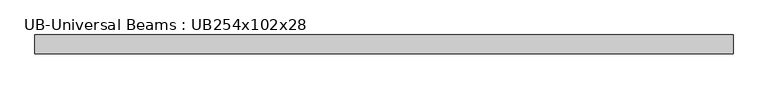
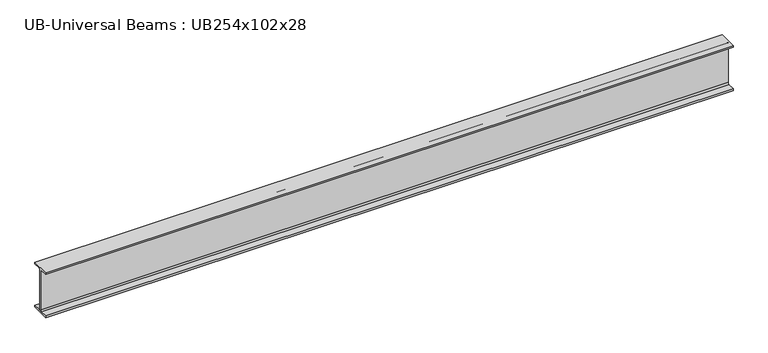
"""IFC4 building model written with IfcOpenShell, lengths in millimetres: beam geometry, UB-Universal Beams : UB254x102x28."""

from ifc_helpers import new_model, si_unit, point, frame, frame_2d, origin, place, context, project, spatial, polyline, circle_curve, trimmed, segment, composite_curve, outline, extrude, source, transform, mapped, element, save


def ub_universal_beams_ub254x102x28_3001bc84(model_context):
    return source(origin(), model_context, "Body", "SweptSolid", [
        extrude(outline(composite_curve([segment(polyline([(51.1, -120.2), (51.1, -130.2), (-51.1, -130.2), (-51.1, -120.2), (-10.75, -120.2)]), True, "CONTINUOUS"), segment(trimmed(circle_curve(frame_2d((-10.75, -112.6)), 7.6), [point((-10.75, -120.2))], [point((-3.15, -112.6))], True, "CARTESIAN"), True, "CONTINUOUS"), segment(polyline([(-3.15, -112.6), (-3.15, 112.6)]), True, "CONTINUOUS"), segment(trimmed(circle_curve(frame_2d((-10.75, 112.6)), 7.6), [point((-3.15, 112.6))], [point((-10.75, 120.2))], True, "CARTESIAN"), True, "CONTINUOUS"), segment(polyline([(-10.75, 120.2), (-51.1, 120.2), (-51.1, 130.2), (51.1, 130.2), (51.1, 120.2), (10.75, 120.2)]), True, "CONTINUOUS"), segment(trimmed(circle_curve(frame_2d((10.75, 112.6)), 7.6), [point((10.75, 120.2))], [point((3.15, 112.6))], True, "CARTESIAN"), True, "CONTINUOUS"), segment(polyline([(3.15, 112.6), (3.15, -112.6)]), True, "CONTINUOUS"), segment(trimmed(circle_curve(frame_2d((10.75, -112.6)), 7.6), [point((3.15, -112.6))], [point((10.75, -120.2))], True, "CARTESIAN"), True, "CONTINUOUS"), segment(polyline([(10.75, -120.2), (51.1, -120.2)]), True, "CONTINUOUS")], self_intersect=False)), frame((-1885.1, 0.0, 0.0), z_axis=(1.0, 0.0, 0.0), x_axis=(0.0, 1.0, 0.0)), (0.0, 0.0, 1.0), 3770.2),
    ])


if __name__ == "__main__":
    model = new_model("IFC4")
    model_context = context("Model", 3, world=origin())
    ifc_project = project(units=[si_unit("LENGTHUNIT", "METRE", prefix="MILLI")], contexts=[model_context])
    site = spatial("IfcSite", under=ifc_project)
    building = spatial("IfcBuilding", under=site)
    placement = place(None, origin())
    ub_universal_beams_ub254x102x28_shape = ub_universal_beams_ub254x102x28_3001bc84(model_context)
    element("IfcBeam", 1, ObjectType="UB-Universal Beams : UB254x102x28", at=placement, inside=building, context=model_context, shape_type="MappedRepresentation", body=[
        mapped(ub_universal_beams_ub254x102x28_shape, transform((0.0, 0.0, 0.0), x_axis=(1.0, 0.0, 0.0), y_axis=(0.0, 1.0, 0.0), z_axis=(0.0, 0.0, 1.0))),
    ])
    save(model, "model.ifc")

# Revit data of these elements
# Type "UB-Universal Beams : UB254x102x28"
#   Section Name Key = "UB254X102X28"
#   Width = 10.22 cm
#   Web Thickness = 0.63 cm
#   Web Fillet = 0.76 cm
#   Warping Constant = 28000.0 cm⁶
#   Torsional Moment of Inertia = 9.57 cm⁴
#   Section Area = 36.1 cm²
#   Plastic Modulus weak axis = 54.8 cm³
#   Plastic Modulus strong axis = 353.0 cm³
#   Nominal Weight = 28.2999 kgf/m
#   Moment of Inertia weak axis = 179.00 cm⁴
#   Moment of Inertia strong axis = 4005.00 cm⁴
#   Height = 26.04 cm
#   Flange Thickness = 1.0 cm
#   Elastic Modulus weak axis = 34.9 cm³
#   Elastic Modulus strong axis = 308.0 cm³
#   Centroid Vertical = 13.02 cm
#   Centroid Horizontal = 5.11 cm
#   Bolt Spacing = 5.4 cm
#   Length [instance default] = 4' - 11.05512"
#   Structural Material [instance default] = Metal - Steel 43-275
#   Type Comments = ""
#   Assembly Code = ""
# Element 1 (IfcBeam, "UB-Universal Beams : UB254x102x28")
#   Materials on its faces: "Metal - Steel 43-275"
# Materials
#   "Metal - Steel 43-275": class "Metal", colour RGB 247 247 247, transparency 0, Cost = 0
